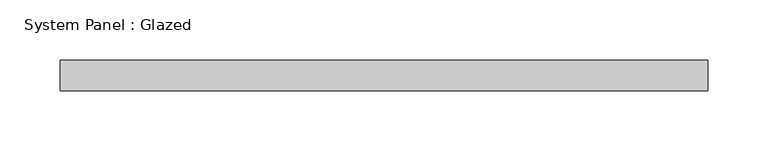
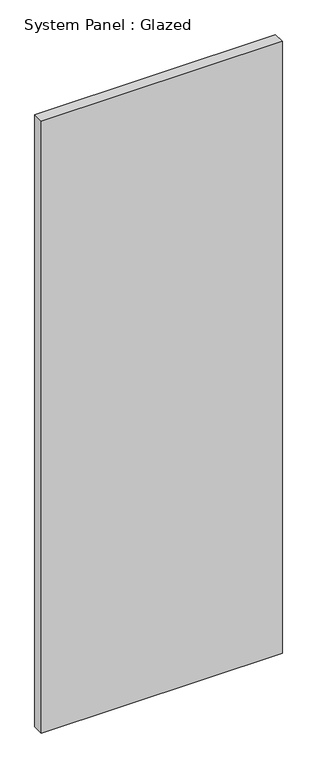
"""IFC4 building model written with IfcOpenShell, lengths in millimetres: plate geometry, System Panel : Glazed."""

from ifc_helpers import new_model, si_unit, origin, origin_with_axes, place, context, project, spatial, polyline, outline, extrude, source, transform, mapped, element, save


def system_panel_glazed_f75ed1c4(model_context):
    return source(origin(), model_context, "Body", "SweptSolid", [
        extrude(outline(polyline([(269.875, 19.05), (-269.875, 19.05), (-269.875, 44.45), (269.875, 44.45), (269.875, 19.05)])), origin_with_axes(), (0.0, 0.0, 1.0), 1448.4674874),
    ])


if __name__ == "__main__":
    model = new_model("IFC4")
    model_context = context("Model", 3, world=origin())
    ifc_project = project(units=[si_unit("LENGTHUNIT", "METRE", prefix="MILLI")], contexts=[model_context])
    site = spatial("IfcSite", under=ifc_project)
    building = spatial("IfcBuilding", under=site)
    placement = place(None, origin())
    system_panel_glazed_shape = system_panel_glazed_f75ed1c4(model_context)
    element("IfcPlate", 1, ObjectType="System Panel : Glazed", at=placement, inside=building, context=model_context, shape_type="MappedRepresentation", body=[
        mapped(system_panel_glazed_shape, transform((0.0, 0.0, 0.0), x_axis=(1.0, 0.0, 0.0), y_axis=(0.0, 1.0, 0.0), z_axis=(0.0, 0.0, 1.0))),
    ])
    save(model, "model.ifc")

# Revit data of these elements
# Type "System Panel : Glazed"
#   Construction Type Id = "GSP4R"
#   Analytic Construction = "1/8 in Pilkington single glazing"
#   Visual Light Transmittance = 0.9
#   Solar Heat Gain Coefficient = 0.86
#   Heat Transfer Coefficient (U) = 1.18115 BTU/(h·ft²·°F)
#   Define Thermal Properties by = 1
# Element 1 (IfcPlate, "System Panel : Glazed")
#   Materials on its faces: "Glass"
# Materials
#   "Glass": class "Glass", colour RGB 0 128 192, transparency 0.75, Description = "Soda Lime Glass", Cost = 0
